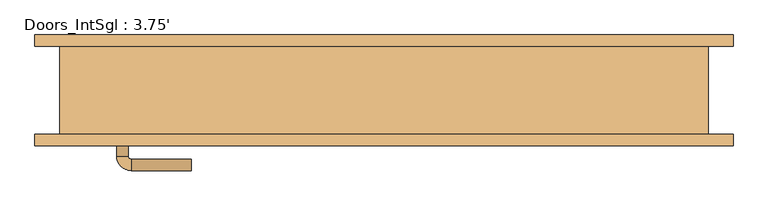
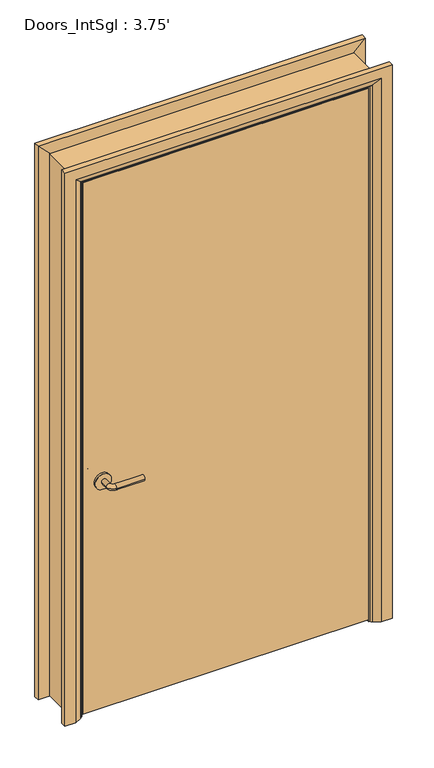
"""IFC4 building model written with IfcOpenShell, lengths in millimetres: door geometry, Doors_IntSgl : 3.75'."""

from ifc_helpers import new_model, si_unit, point, frame, frame_2d, origin, place, context, project, spatial, polyline, circle_curve, ellipse_curve, trimmed, segment, composite_curve, outline, extrude, faceted_brep, source, transform, mapped, element, save
from ifc_brep_helpers import plane_surface, cylinder_surface, revolved_surface, advanced_brep


def doors_intsgl_3_75_1d728d0e(model_context):
    return source(origin(), model_context, "Body", "SolidModel", [
        advanced_brep(
        [(-464.5, -30.2, 900.0), (-444.5, -30.2, 900.0), (-464.5, -0.2, 900.0), (-444.5, -0.2, 900.0), (-439.5, 4.8, 900.0), (-439.5, 24.8, 900.0), (-334.5, 24.8, 900.0), (-334.5, 4.8, 900.0)],
        [
            (0, 1, circle_curve(frame((-454.5, -30.2, 900.0), z_axis=(0.0, -1.0, 0.0), x_axis=(1.0, 0.0, 0.0)), 10.0)),
            (1, 0, circle_curve(frame((-454.5, -30.2, 900.0), z_axis=(0.0, -1.0, 0.0), x_axis=(1.0, 0.0, 0.0)), 10.0)),
            (0, 2),
            (2, 3, circle_curve(frame((-454.5, -0.2, 900.0), z_axis=(0.0, -1.0, 0.0), x_axis=(1.0, 0.0, 0.0)), 10.0)),
            (3, 1),
            (3, 2, circle_curve(frame((-454.5, -0.2, 900.0), z_axis=(0.0, -1.0, 0.0), x_axis=(1.0, 0.0, 0.0)), 10.0)),
            (4, 3, circle_curve(frame((-439.5, -0.2, 900.0), z_axis=(0.0, 0.0, 1.0), x_axis=(-1.0, 0.0, 0.0)), 5.0)),
            (2, 5, circle_curve(frame((-439.5, -0.2, 900.0), z_axis=(0.0, 0.0, -1.0), x_axis=(-1.0, 0.0, 0.0)), 25.0)),
            (5, 4, circle_curve(frame((-439.5, 14.8, 900.0), z_axis=(-1.0, 0.0, 0.0), x_axis=(0.0, -1.0, 0.0)), 10.0)),
            (4, 5, circle_curve(frame((-439.5, 14.8, 900.0), z_axis=(-1.0, 0.0, 0.0), x_axis=(0.0, -1.0, 0.0)), 10.0)),
            (6, 7, circle_curve(frame((-334.5, 14.8, 900.0), z_axis=(1.0, 0.0, 0.0), x_axis=(0.0, -1.0, 0.0)), 10.0)),
            (7, 6, circle_curve(frame((-334.5, 14.8, 900.0), z_axis=(1.0, 0.0, 0.0), x_axis=(0.0, -1.0, 0.0)), 10.0)),
            (5, 6),
            (7, 4),
        ],
        [
            plane_surface(frame((-454.5, -30.2, 900.0), z_axis=(0.0, -1.0, 0.0), x_axis=(0.0, 0.0, 1.0))),
            cylinder_surface(frame((-454.5, -30.2, 900.0), z_axis=(0.0, -1.0, 0.0), x_axis=(1.0, 0.0, 0.0)), 10.0),
            revolved_surface(trimmed(ellipse_curve(frame((-454.5, -0.2, 900.0), z_axis=(0.0, -1.0, 0.0), x_axis=(1.0, 0.0, 0.0)), 10.0, 10.0), [point((-464.5, -0.2, 900.0))], [point((-444.5, -0.2, 900.0))], True, "CARTESIAN"), (-439.5, -0.2, 900.0), (0.0, 0.0, -1.0)),
            revolved_surface(trimmed(ellipse_curve(frame((-454.5, -0.2, 900.0), z_axis=(0.0, -1.0, 0.0), x_axis=(1.0, 0.0, 0.0)), 10.0, 10.0), [point((-444.5, -0.2, 900.0))], [point((-464.5, -0.2, 900.0))], True, "CARTESIAN"), (-439.5, -0.2, 900.0), (0.0, 0.0, -1.0)),
            plane_surface(frame((-334.5, 14.8, 900.0), z_axis=(1.0, 0.0, 0.0), x_axis=(0.0, 0.0, 1.0))),
            cylinder_surface(frame((-439.5, 14.8, 900.0), z_axis=(-1.0, 0.0, 0.0), x_axis=(0.0, -1.0, 0.0)), 10.0),
        ],
        [
            (0, [[1, 2]]),
            (1, [[-1, 3, 4, 5]]),
            (1, [[-2, -5, 6, -3]]),
            (2, [[7, -4, 8, 9]]),
            (3, [[-8, -6, -7, 10]]),
            (4, [[11, 12]]),
            (5, [[-9, 13, -12, 14]]),
            (5, [[-10, -14, -11, -13]]),
        ],
    ),
        extrude(outline(composite_curve([segment(trimmed(circle_curve(frame_2d((900.0, -457.0)), 30.0), [point((900.0, -487.0))], [point((900.0, -427.0))], False, "CARTESIAN"), True, "CONTINUOUS"), segment(trimmed(circle_curve(frame_2d((900.0, -457.0)), 30.0), [point((900.0, -427.0))], [point((900.0, -487.0))], False, "CARTESIAN"), True, "CONTINUOUS")], self_intersect=False)), frame((0.0, -38.2, 0.0), z_axis=(0.0, 1.0, 0.0), x_axis=(0.0, 0.0, 1.0)), (0.0, 0.0, 1.0), 8.0),
        advanced_brep(
        [(-464.5, -84.2, 900.0), (-444.5, -84.2, 900.0), (-444.5, -114.2, 900.0), (-464.5, -114.2, 900.0), (-439.5, -119.2, 900.0), (-439.5, -139.2, 900.0), (-334.5, -139.2, 900.0), (-334.5, -119.2, 900.0)],
        [
            (0, 1, circle_curve(frame((-454.5, -84.2, 900.0), z_axis=(0.0, 1.0, 0.0), x_axis=(1.0, 0.0, 0.0)), 10.0)),
            (1, 0, circle_curve(frame((-454.5, -84.2, 900.0), z_axis=(0.0, 1.0, 0.0), x_axis=(1.0, 0.0, 0.0)), 10.0)),
            (1, 2),
            (2, 3, circle_curve(frame((-454.5, -114.2, 900.0), z_axis=(0.0, 1.0, 0.0), x_axis=(1.0, 0.0, 0.0)), 10.0)),
            (3, 0),
            (3, 2, circle_curve(frame((-454.5, -114.2, 900.0), z_axis=(0.0, 1.0, 0.0), x_axis=(1.0, 0.0, 0.0)), 10.0)),
            (4, 5, circle_curve(frame((-439.5, -129.2, 900.0), z_axis=(-1.0, 0.0, 0.0), x_axis=(0.0, 1.0, 0.0)), 10.0)),
            (5, 3, circle_curve(frame((-439.5, -114.2, 900.0), z_axis=(0.0, 0.0, -1.0), x_axis=(-1.0, 0.0, 0.0)), 25.0)),
            (2, 4, circle_curve(frame((-439.5, -114.2, 900.0), z_axis=(0.0, 0.0, 1.0), x_axis=(-1.0, 0.0, 0.0)), 5.0)),
            (5, 4, circle_curve(frame((-439.5, -129.2, 900.0), z_axis=(-1.0, 0.0, 0.0), x_axis=(0.0, 1.0, 0.0)), 10.0)),
            (6, 7, circle_curve(frame((-334.5, -129.2, 900.0), z_axis=(1.0, 0.0, 0.0), x_axis=(0.0, 1.0, 0.0)), 10.0)),
            (7, 6, circle_curve(frame((-334.5, -129.2, 900.0), z_axis=(1.0, 0.0, 0.0), x_axis=(0.0, 1.0, 0.0)), 10.0)),
            (4, 7),
            (6, 5),
        ],
        [
            plane_surface(frame((-454.5, -84.2, 900.0), z_axis=(0.0, 1.0, 0.0), x_axis=(0.0, 0.0, 1.0))),
            cylinder_surface(frame((-454.5, -84.2, 900.0), z_axis=(0.0, 1.0, 0.0), x_axis=(1.0, 0.0, 0.0)), 10.0),
            revolved_surface(trimmed(ellipse_curve(frame((-454.5, -114.2, 900.0), z_axis=(0.0, -1.0, 0.0), x_axis=(1.0, 0.0, 0.0)), 10.0, 10.0), [point((-464.5, -114.2, 900.0))], [point((-444.5, -114.2, 900.0))], True, "CARTESIAN"), (-439.5, -114.2, 900.0), (0.0, 0.0, -1.0)),
            revolved_surface(trimmed(ellipse_curve(frame((-454.5, -114.2, 900.0), z_axis=(0.0, -1.0, 0.0), x_axis=(1.0, 0.0, 0.0)), 10.0, 10.0), [point((-444.5, -114.2, 900.0))], [point((-464.5, -114.2, 900.0))], True, "CARTESIAN"), (-439.5, -114.2, 900.0), (0.0, 0.0, -1.0)),
            plane_surface(frame((-334.5, -129.2, 900.0), z_axis=(1.0, 0.0, 0.0), x_axis=(0.0, 0.0, 1.0))),
            cylinder_surface(frame((-439.5, -129.2, 900.0), z_axis=(-1.0, 0.0, 0.0), x_axis=(0.0, 1.0, 0.0)), 10.0),
        ],
        [
            (0, [[1, 2]]),
            (1, [[3, 4, 5, -2]]),
            (1, [[-5, 6, -3, -1]]),
            (2, [[7, 8, -4, 9]]),
            (3, [[10, -9, -6, -8]]),
            (4, [[11, 12]]),
            (5, [[13, -11, 14, -7]]),
            (5, [[-14, -12, -13, -10]]),
        ],
    ),
        extrude(outline(composite_curve([segment(trimmed(circle_curve(frame_2d((900.0, -457.0)), 30.0), [point((900.0, -487.0))], [point((900.0, -427.0))], False, "CARTESIAN"), True, "CONTINUOUS"), segment(trimmed(circle_curve(frame_2d((900.0, -457.0)), 30.0), [point((900.0, -427.0))], [point((900.0, -487.0))], False, "CARTESIAN"), True, "CONTINUOUS")], self_intersect=False)), frame((0.0, -84.2, 0.0), z_axis=(0.0, 1.0, 0.0), x_axis=(0.0, 0.0, 1.0)), (0.0, 0.0, 1.0), 8.0),
        extrude(outline(polyline([(529.5, -38.2), (529.5, -76.2), (-529.5, -76.2), (-529.5, -38.2), (529.5, -38.2)])), frame((0.0, 0.0, 8.0), z_axis=(0.0, 0.0, 1.0), x_axis=(1.0, 0.0, 0.0)), (0.0, 0.0, 1.0), 2083.6),
        advanced_brep(
        [(606.5, -96.2, 0.0), (566.5, -96.2, 0.0), (540.5, -82.2, 0.0), (536.5, -76.2, 0.0), (606.5, -76.2, 0.0), (606.5, -76.2, 2168.6), (606.5, -96.2, 2168.6), (536.5, -76.2, 2098.6), (-536.5, -76.2, 2098.6), (-536.5, -76.2, 0.0), (-606.5, -76.2, 0.0), (-606.5, -76.2, 2168.6), (540.5, -82.2, 2102.6), (566.5, -96.2, 2128.6), (-606.5, -96.2, 2168.6), (-606.5, -96.2, 0.0), (-566.5, -96.2, 0.0), (-566.5, -96.2, 2128.6), (-540.5, -82.2, 0.0), (-540.5, -82.2, 2102.6)],
        [
            (0, 1),
            (1, 2),
            (2, 3, circle_curve(frame((544.5, -75.2, 0.0), z_axis=(0.0, 0.0, -1.0), x_axis=(1.0, 0.0, 0.0)), 8.0622577)),
            (3, 4),
            (4, 0),
            (4, 5),
            (5, 6),
            (6, 0),
            (3, 7),
            (7, 8),
            (8, 9),
            (9, 10),
            (10, 11),
            (11, 5),
            (2, 12),
            (12, 7, ellipse_curve(frame((544.5, -75.2, 2106.6), z_axis=(0.7071067811865475, 0.0, -0.7071067811865475), x_axis=(-0.7071067811865474, 0.0, -0.7071067811865476)), 11.4017543, 8.0622577)),
            (1, 13),
            (13, 12),
            (6, 14),
            (14, 15),
            (15, 16),
            (16, 17),
            (17, 13),
            (10, 15),
            (14, 11),
            (9, 18, circle_curve(frame((-544.5, -75.2, 0.0), z_axis=(0.0, 0.0, -1.0), x_axis=(-1.0, 0.0, 0.0)), 8.0622577)),
            (18, 16),
            (19, 18),
            (8, 19, ellipse_curve(frame((-544.5, -75.2, 2106.6), z_axis=(-0.7071067811865475, 0.0, -0.7071067811865475), x_axis=(-0.7071067811865474, 0.0, 0.7071067811865476)), 11.4017543, 8.0622577)),
            (19, 17),
            (12, 19),
        ],
        [
            plane_surface(frame((536.5, -76.2, 0.0), z_axis=(0.0, 0.0, -1.0), x_axis=(0.0, 1.0, 0.0))),
            plane_surface(frame((606.5, -96.2, 0.0), z_axis=(1.0, 0.0, 0.0), x_axis=(0.0, 0.0, 1.0))),
            plane_surface(frame((606.5, -76.2, 0.0), z_axis=(0.0, 1.0, 0.0), x_axis=(0.0, 0.0, 1.0))),
            cylinder_surface(frame((544.5, -75.2, 0.0), z_axis=(0.0, 0.0, -1.0), x_axis=(1.0, 0.0, 0.0)), 8.0622577),
            plane_surface(frame((540.5, -82.2, 0.0), z_axis=(-0.4740998230350126, -0.880471099922178, 0.0), x_axis=(0.0, 0.0, 1.0))),
            plane_surface(frame((566.5, -96.2, 0.0), z_axis=(0.0, -1.0, 0.0), x_axis=(0.0, 0.0, 1.0))),
            plane_surface(frame((-606.5, -96.2, 2168.6), z_axis=(-1.0, 0.0, 0.0), x_axis=(0.0, 0.0, -1.0))),
            plane_surface(frame((-536.5, -76.2, 0.0), z_axis=(0.0, 0.0, -1.0), x_axis=(0.0, 1.0, 0.0))),
            cylinder_surface(frame((-544.5, -75.2, 2098.6), z_axis=(0.0, 0.0, 1.0), x_axis=(-1.0, 0.0, 0.0)), 8.0622577),
            plane_surface(frame((-540.5, -82.2, 2102.6), z_axis=(0.47409982303501824, -0.8804710999221749, 0.0), x_axis=(0.0, 0.0, -1.0))),
            plane_surface(frame((606.5, -96.2, 2168.6), z_axis=(0.0, 0.0, 1.0), x_axis=(-1.0, 0.0, 0.0))),
            cylinder_surface(frame((536.5, -75.2, 2106.6), z_axis=(1.0, 0.0, 0.0), x_axis=(0.0, 0.0, 1.0)), 8.0622577),
            plane_surface(frame((540.5, -82.2, 2102.6), z_axis=(0.0, -0.8804710999221764, -0.4740998230350154), x_axis=(-1.0, 0.0, 0.0))),
        ],
        [
            (0, [[1, 2, 3, 4, 5]]),
            (1, [[6, 7, 8, -5]]),
            (2, [[9, 10, 11, 12, 13, 14, -6, -4]]),
            (3, [[15, 16, -9, -3]]),
            (4, [[17, 18, -15, -2]]),
            (5, [[-8, 19, 20, 21, 22, 23, -17, -1]]),
            (6, [[-13, 24, -20, 25]]),
            (7, [[-24, -12, 26, 27, -21]]),
            (8, [[28, -26, -11, 29]]),
            (9, [[-22, -27, -28, 30]]),
            (10, [[-14, -25, -19, -7]]),
            (11, [[31, -29, -10, -16]]),
            (12, [[-23, -30, -31, -18]]),
        ],
    ),
        extrude(outline(polyline([(0.0, -512.5), (2074.6, -512.5), (2074.6, 512.5), (0.0, 512.5), (0.0, 531.5), (2093.6, 531.5), (2093.6, -531.5), (0.0, -531.5), (0.0, -512.5)])), frame((0.0, -36.2, 0.0), z_axis=(0.0, 1.0, 0.0), x_axis=(0.0, 0.0, 1.0)), (0.0, 0.0, 1.0), 32.0),
        advanced_brep(
        [(-606.5, 96.2, 0.0), (-566.5, 96.2, 0.0), (-540.5, 82.2, 0.0), (-536.5, 76.2, 0.0), (-606.5, 76.2, 0.0), (-606.5, 76.2, 2168.6), (-606.5, 96.2, 2168.6), (-536.5, 76.2, 2098.6), (-540.5, 82.2, 2102.6), (-566.5, 96.2, 2128.6), (606.5, 96.2, 0.0), (606.5, 76.2, 0.0), (536.5, 76.2, 0.0), (540.5, 82.2, 0.0), (566.5, 96.2, 0.0), (606.5, 96.2, 2168.6), (566.5, 96.2, 2128.6), (540.5, 82.2, 2102.6), (536.5, 76.2, 2098.6), (606.5, 76.2, 2168.6)],
        [
            (0, 1),
            (1, 2),
            (2, 3, circle_curve(frame((-544.5, 75.2, 0.0), z_axis=(0.0, 0.0, -1.0), x_axis=(-1.0, 0.0, 0.0)), 8.0622577)),
            (3, 4),
            (4, 0),
            (4, 5),
            (5, 6),
            (6, 0),
            (3, 7),
            (7, 5),
            (2, 8),
            (8, 7, ellipse_curve(frame((-544.5, 75.2, 2106.6), z_axis=(-0.7071067811865475, 0.0, -0.7071067811865475), x_axis=(0.7071067811865474, 0.0, -0.7071067811865476)), 11.4017543, 8.0622577)),
            (1, 9),
            (9, 8),
            (6, 9),
            (10, 11),
            (11, 12),
            (12, 13, circle_curve(frame((544.5, 75.2, 0.0), z_axis=(0.0, 0.0, -1.0), x_axis=(1.0, 0.0, 0.0)), 8.0622577)),
            (13, 14),
            (14, 10),
            (15, 10),
            (14, 16),
            (16, 15),
            (13, 17),
            (17, 16),
            (12, 18),
            (18, 17, ellipse_curve(frame((544.5, 75.2, 2106.6), z_axis=(0.7071067811865475, 0.0, -0.7071067811865475), x_axis=(0.7071067811865474, 0.0, 0.7071067811865476)), 11.4017543, 8.0622577)),
            (11, 19),
            (19, 18),
            (15, 19),
            (5, 19),
            (15, 6),
            (7, 18),
            (8, 17),
            (9, 16),
        ],
        [
            plane_surface(frame((-536.5, 149.0010989, 0.0), z_axis=(0.0, 0.0, -1.0), x_axis=(1.0, 0.0, 0.0))),
            plane_surface(frame((-606.5, 96.2, 0.0), z_axis=(-1.0, 0.0, 0.0), x_axis=(0.0, 0.0, 1.0))),
            plane_surface(frame((-606.5, 76.2, 0.0), z_axis=(0.0, -1.0, 0.0), x_axis=(0.0, 0.0, 1.0))),
            cylinder_surface(frame((-544.5, 75.2, 0.0), z_axis=(0.0, 0.0, -1.0), x_axis=(-1.0, 0.0, 0.0)), 8.0622577),
            plane_surface(frame((-540.5, 82.2, 0.0), z_axis=(0.4740998230350183, 0.8804710999221749, 0.0), x_axis=(0.0, 0.0, 1.0))),
            plane_surface(frame((-566.5, 96.2, 0.0), z_axis=(0.0, 1.0, 0.0), x_axis=(0.0, 0.0, 1.0))),
            plane_surface(frame((536.5, 149.0010989, 0.0), z_axis=(0.0, 0.0, -1.0), x_axis=(-1.0, 0.0, 0.0))),
            plane_surface(frame((566.5, 96.2, 2128.6), z_axis=(0.0, 1.0, 0.0), x_axis=(0.0, 0.0, -1.0))),
            plane_surface(frame((540.5, 82.2, 2102.6), z_axis=(-0.4740998230350183, 0.8804710999221749, 0.0), x_axis=(0.0, 0.0, -1.0))),
            cylinder_surface(frame((544.5, 75.2, 2098.6), z_axis=(0.0, 0.0, 1.0), x_axis=(1.0, 0.0, 0.0)), 8.0622577),
            plane_surface(frame((606.5, 76.2, 2168.6), z_axis=(0.0, -1.0, 0.0), x_axis=(0.0, 0.0, -1.0))),
            plane_surface(frame((606.5, 96.2, 2168.6), z_axis=(1.0, 0.0, 0.0), x_axis=(0.0, 0.0, -1.0))),
            plane_surface(frame((-606.5, 96.2, 2168.6), z_axis=(0.0, 0.0, 1.0), x_axis=(1.0, 0.0, 0.0))),
            plane_surface(frame((-606.5, 76.2, 2168.6), z_axis=(0.0, -1.0, 0.0), x_axis=(1.0, 0.0, 0.0))),
            cylinder_surface(frame((-536.5, 75.2, 2106.6), z_axis=(-1.0, 0.0, 0.0), x_axis=(0.0, 0.0, 1.0)), 8.0622577),
            plane_surface(frame((-540.5, 82.2, 2102.6), z_axis=(0.0, 0.8804710999221749, -0.4740998230350183), x_axis=(1.0, 0.0, 0.0))),
            plane_surface(frame((-566.5, 96.2, 2128.6), z_axis=(0.0, 1.0, 0.0), x_axis=(1.0, 0.0, 0.0))),
        ],
        [
            (0, [[1, 2, 3, 4, 5]]),
            (1, [[6, 7, 8, -5]]),
            (2, [[9, 10, -6, -4]]),
            (3, [[11, 12, -9, -3]]),
            (4, [[13, 14, -11, -2]]),
            (5, [[-8, 15, -13, -1]]),
            (6, [[16, 17, 18, 19, 20]]),
            (7, [[21, -20, 22, 23]]),
            (8, [[-22, -19, 24, 25]]),
            (9, [[-24, -18, 26, 27]]),
            (10, [[-26, -17, 28, 29]]),
            (11, [[-28, -16, -21, 30]]),
            (12, [[31, -30, 32, -7]]),
            (13, [[33, -29, -31, -10]]),
            (14, [[34, -27, -33, -12]]),
            (15, [[35, -25, -34, -14]]),
            (16, [[-32, -23, -35, -15]]),
        ],
    ),
        faceted_brep([(-531.5, -76.2, 0.0), (-563.5, -76.2, 0.0), (-563.5, 76.2, 0.0), (-531.5, 76.2, 0.0), (-531.5, 76.2, 2093.6), (-531.5, -76.2, 2093.6), (-563.5, 76.2, 2125.6), (-563.5, -76.2, 2125.6), (531.5, -76.2, 0.0), (531.5, 76.2, 0.0), (563.5, 76.2, 0.0), (563.5, -76.2, 0.0), (531.5, -76.2, 2093.6), (563.5, -76.2, 2125.6), (563.5, 76.2, 2125.6), (531.5, 76.2, 2093.6)], [[[0, 1, 2, 3]], [[3, 4, 5, 0]], [[2, 6, 4, 3]], [[1, 7, 6, 2]], [[0, 5, 7, 1]], [[8, 9, 10, 11]], [[12, 8, 11, 13]], [[13, 11, 10, 14]], [[14, 10, 9, 15]], [[15, 9, 8, 12]], [[4, 15, 12, 5]], [[6, 14, 15, 4]], [[7, 13, 14, 6]], [[5, 12, 13, 7]]]),
    ])


if __name__ == "__main__":
    model = new_model("IFC4")
    model_context = context("Model", 3, world=origin())
    ifc_project = project(units=[si_unit("LENGTHUNIT", "METRE", prefix="MILLI")], contexts=[model_context])
    site = spatial("IfcSite", under=ifc_project)
    building = spatial("IfcBuilding", under=site)
    placement = place(None, origin())
    doors_intsgl_3_75_shape = doors_intsgl_3_75_1d728d0e(model_context)
    element("IfcDoor", 1, ObjectType="Doors_IntSgl : 3.75'", at=placement, inside=building, context=model_context, shape_type="MappedRepresentation", body=[
        mapped(doors_intsgl_3_75_shape, transform((0.0, 0.0, 0.0), x_axis=(1.0, 0.0, 0.0), y_axis=(0.0, 1.0, 0.0), z_axis=(0.0, 0.0, 1.0))),
    ])
    save(model, "model.ifc")

# Revit data of these elements
# Type "Doors_IntSgl : 3.75'"
#   Type Mark = "58"
#   Type Comments = "Internal Single"
#   Operation = "SingleSwingRight"
#   Manufacturer = "Revit"
#   Keynote = "L20"
#   Description = "Internal Single Door"
#   Analytic Construction = "Metal"
#   UnderCut = 8 mm
#   Tolerance = 2 mm
#   Thickness = 38 mm
#   Thermal Resistance (R) = 0.270117 (m²·K)/W
#   Structural Tolerance = 8 mm
#   StopDepth = 32 mm
#   Stop Thickness = 19 mm
#   Rough Width = 1143 mm
#   Rough Height = 2133.6 mm
#   Height to Top Lock Rail = 1000 mm
#   Heat Transfer Coefficient (U) = 3.7021 W/(m²·K)
#   Handle Z Distance = 900 mm
#   Handle X Distance = 75 mm
#   Frame Thickness = 32 mm
#   Door Panel Width = 1059 mm
#   Door Panel Thickness = 38 mm
#   Door Panel Offset = 0 mm
#   Height = 2133.6 mm
#   Width = 1143 mm
#   Door Panel Height = 2083.6 mm
#   Architrave Setback = 5 mm
#   Vis - Ironmongery = yes
#   Material Ironmongery = Door - Handle
#   Material Frame = Door - Frame/Mullion (1)
#   Material Door = Door - Panel
#   Material Architrave = Door - Architrave
#   Visual Light Transmittance = 0
#   Solar Heat Gain Coefficient = 0
#   Function = (empty or 0)
#   Wall Closure = (empty or 0)
# Element 1 (IfcDoor, "Doors_IntSgl : 3.75'")
#   Materials on its faces: "Door - Architrave", "Door - Handle", "Door - Frame/Mullion (1)", "Door - Panel"
# Materials
#   "Door - Handle": colour RGB 0 0 0, transparency 0, Keynote = "P21", Cost = 0
#   "Door - Frame/Mullion (1)": class "Wood", colour RGB 212 179 113, transparency 0, Keynote = "L20", Cost = 0
#   "Door - Panel": class "Wood", colour RGB 210 159 95, transparency 0, Keynote = "L20", Cost = 0
#   "Door - Architrave": class "Wood", colour RGB 154 90 5, transparency 0, Keynote = "P20", Cost = 0
